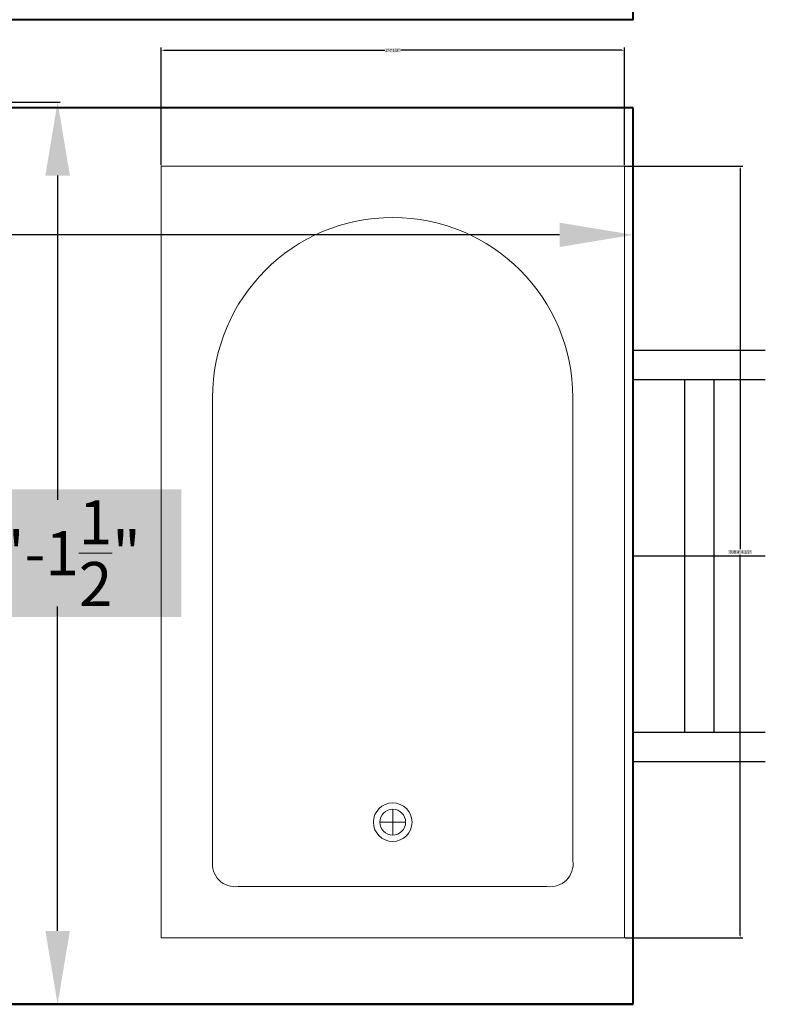
# Model space of a CAD drawing. Units: inches. Extents: x -301 to 715, y -607 to 364.
# Tile 98 of 141: x 82 to 133, y -77 to -10. Entities that reach past the tile are written whole.
import ezdxf

# ---------------------------------------------------------------- set-up
doc = ezdxf.new("R2010")
doc.units = ezdxf.units.IN
doc.header["$MEASUREMENT"] = 0
for name, color, linetype, lineweight in [('A-ANNO-DIMS', 2, 'Continuous', 18), ('A-FLOR-FIXT', 9, 'Continuous', 18), ('A-GLAZ', 2, 'Continuous', 25), ('A-WALL', 3, 'Continuous', 40)]:
    doc.layers.add(name, color=color, linetype=linetype, lineweight=lineweight)
doc.styles.get("Standard").update_dxf_attribs({"font": 'arial.ttf'})
doc.dimstyles.get("Standard").update_dxf_attribs({"dimtxt": 0.18, "dimasz": 0.18, "dimexe": 0.18, "dimexo": 0.0625, "dimgap": 0.09, "dimtad": 0, "dimtih": 1, "dimtoh": 1, "dimdec": 1, "dimzin": 0, "dimdsep": 46, "dimlunit": 4, "dimtxsty": 'Standard', "dimcen": 0.09, "dimclrd": 3, "dimclre": 4, "dimclrt": 6, "dimadec": 0, "dimazin": 0, "dimtfac": 1, "dimtdec": 1, "dimtofl": 0, "dimtmove": 0, "dimatfit": 3, "dimfxl": 1, "dimtfill": 2, "dimtfillclr": 51, "dimtolj": 1, "dimtzin": 0, "dimarcsym": 0})

# ---------------------------------------------------------------- blocks, each defined once
blk = doc.blocks.new('Bath Tub - 26 x 60 in.')
for p, q in [((9, -17), (9, -19)), ((8, -18), (10, -18))]:
    blk.add_line(p, q)
blk.add_lwpolyline([(0, -36), (0, 0), (60, 0), (60, -36)], close=True)
for points in [[(6, -4), (42, -4)], [(4, -30), (4, -6)], [(42, -32), (6, -32)]]:
    blk.add_lwpolyline(points)
for radius in [1.5, 1]:
    blk.add_circle((9, -18), radius)
for centre, radius, start, end in [((5.75, -5.75), 1.768, 81.8699, 188.1301), ((42, -18), 14, 270, 90), ((5.75, -30.25), 1.768, 171.8699, 278.1301)]:
    blk.add_arc(centre, radius, start, end)
blk = doc.blocks.new('*D46')
at = {"layer": 'A-ANNO-DIMS', "color": 0, "lineweight": -2, "transparency": 16777216}
for p, q in [((27.897, -15.88), (27.897, -24.639)), ((123.897, -15.88), (123.897, -24.639)), ((32.897, -24.459), (74.424, -24.459)), ((118.897, -24.459), (77.369, -24.459))]:
    blk.add_line(p, q, dxfattribs=at)
at = {"layer": 'A-ANNO-DIMS', "color": 0, "transparency": 16777216}
for points in [[(32.897, -23.626), (32.897, -25.292), (27.897, -24.459)], [(118.897, -23.626), (118.897, -25.292), (123.897, -24.459)]]:
    blk.add_solid(points, dxfattribs=at)
at = {"layer": 'Defpoints', "color": 0, "transparency": 16777216}
for p in [(27.897, -15.818), (123.897, -15.818), (123.897, -24.459)]:
    blk.add_point(p, dxfattribs=at)
at = {"layer": 'A-ANNO-DIMS', "color": 0, "transparency": 16777216, "insert": (75.897, -24.459), "char_height": 3, "attachment_point": 5, "bg_fill": 1, "box_fill_scale": 1.25, "bg_fill_color": 51, "bg_fill_transparency": 0}
blk.add_mtext("\\A1;8'", dxfattribs=at)
blk = doc.blocks.new('*D47')
at = {"layer": 'A-ANNO-DIMS', "color": 0, "lineweight": -2, "transparency": 16777216}
for p, q in [((53.666, -15.423), (84.935, -15.423)), ((84.755, -20.423), (84.755, -42.492)), ((84.755, -71.818), (84.755, -49.748)), ((57.415, -76.818), (84.935, -76.818))]:
    blk.add_line(p, q, dxfattribs=at)
at = {"layer": 'A-ANNO-DIMS', "color": 0, "transparency": 16777216}
for points in [[(83.922, -20.423), (85.588, -20.423), (84.755, -15.423)], [(83.922, -71.818), (85.588, -71.818), (84.755, -76.818)]]:
    blk.add_solid(points, dxfattribs=at)
at = {"layer": 'Defpoints', "color": 0, "transparency": 16777216}
for p in [(53.604, -15.423), (84.755, -15.423), (57.352, -76.818)]:
    blk.add_point(p, dxfattribs=at)
at = {"layer": 'A-ANNO-DIMS', "color": 0, "transparency": 16777216, "insert": (84.755, -46.12), "char_height": 3, "attachment_point": 5, "bg_fill": 1, "box_fill_scale": 1.25, "bg_fill_color": 51, "bg_fill_transparency": 0}
blk.add_mtext('\\A1;5\'-1{\\H1x;\\S1/2;}"', dxfattribs=at)
blk = doc.blocks.new('VENT-24-PLAN')
for p, q in [((0, 0), (0, 9)), ((2, 0), (2, 9)), ((14, 0), (14, 9)), ((26, 0), (26, 9)), ((28, 0), (28, 9)), ((26, 5.5), (2, 5.5)), ((26, 3.5), (2, 3.5))]:
    blk.add_line(p, q)
blk = doc.blocks.new('*D124')
at = {"layer": 'A-ANNO-DIMS', "color": 4, "lineweight": -2, "transparency": 16777216}
for p, q in [((123.372, -19.776), (131.368, -19.776)), ((123.372, -72.302), (131.368, -72.302))]:
    blk.add_line(p, q, dxfattribs=at)
at = {"layer": 'A-ANNO-DIMS', "color": 3, "lineweight": -2, "transparency": 16777216}
for p, q in [((131.188, -19.956), (131.188, -45.856)), ((131.188, -72.122), (131.188, -46.222))]:
    blk.add_line(p, q, dxfattribs=at)
at = {"layer": 'A-ANNO-DIMS', "color": 3, "transparency": 16777216}
for points in [[(131.158, -19.956), (131.218, -19.956), (131.188, -19.776)], [(131.158, -72.122), (131.218, -72.122), (131.188, -72.302)]]:
    blk.add_solid(points, dxfattribs=at)
at = {"layer": 'Defpoints', "color": 0, "transparency": 16777216}
for p in [(123.309, -19.776), (131.188, -19.776), (123.309, -72.302)]:
    blk.add_point(p, dxfattribs=at)
at = {"layer": 'A-ANNO-DIMS', "color": 6, "transparency": 16777216, "insert": (131.188, -46.039), "char_height": 0.18, "attachment_point": 5, "bg_fill": 1, "box_fill_scale": 1.25, "bg_fill_color": 51, "bg_fill_transparency": 0}
blk.add_mtext('\\A1;TUB 4\'-4 1/2"', dxfattribs=at)
blk = doc.blocks.new('*D125')
at = {"layer": 'A-ANNO-DIMS', "color": 4, "lineweight": -2, "transparency": 16777216}
for p, q in [((91.794, -19.714), (91.794, -11.718)), ((123.309, -19.714), (123.309, -11.718))]:
    blk.add_line(p, q, dxfattribs=at)
at = {"layer": 'A-ANNO-DIMS', "color": 3, "lineweight": -2, "transparency": 16777216}
for p, q in [((91.974, -11.898), (107.011, -11.898)), ((123.129, -11.898), (108.092, -11.898))]:
    blk.add_line(p, q, dxfattribs=at)
at = {"layer": 'A-ANNO-DIMS', "color": 3, "transparency": 16777216}
for points in [[(91.974, -11.868), (91.974, -11.928), (91.794, -11.898)], [(123.129, -11.868), (123.129, -11.928), (123.309, -11.898)]]:
    blk.add_solid(points, dxfattribs=at)
at = {"layer": 'Defpoints', "color": 0, "transparency": 16777216}
for p in [(91.794, -11.898), (91.794, -19.776), (123.309, -19.776)]:
    blk.add_point(p, dxfattribs=at)
at = {"layer": 'A-ANNO-DIMS', "color": 6, "transparency": 16777216, "insert": (107.551, -11.898), "char_height": 0.18, "attachment_point": 5, "bg_fill": 1, "box_fill_scale": 1.25, "bg_fill_color": 51, "bg_fill_transparency": 0}
blk.add_mtext('\\A1;2\'-7 1/2"', dxfattribs=at)

msp = doc.modelspace()

# ---------------------------------------------------------------- linework, layer by layer
at = {"layer": 'A-WALL'}
for p, q in [((123.897, -9.818), (123.897, 193.182)), ((123.897, -9.818), (21.897, -9.818)), ((123.897, -15.818), (27.897, -15.818)), ((123.897, -76.818), (123.897, -15.818)), ((57.352, -76.818), (123.897, -76.818)), ((123.897, -76.818), (75.897, -76.818))]:
    msp.add_line(p, q, dxfattribs=at)

# ---------------------------------------------------------------- block references
at = {"layer": 'A-FLOR-FIXT', "xscale": 0.875426725639565, "yscale": 0.875426725639565, "zscale": 0.875426725639565, "rotation": 90}
msp.add_blockref('Bath Tub - 26 x 60 in.', (91.794, -72.302), dxfattribs=at)
at = {"layer": 'A-GLAZ', "rotation": 89.99999999999955}
msp.add_blockref('VENT-24-PLAN', (132.897, -60.318), dxfattribs=at)

# ---------------------------------------------------------------- dimensions: what is measured, and where the dimension line sits
at = {"layer": 'A-ANNO-DIMS'}
for base, p1, p2, angle, override, picture, middle in [((91.794, -11.898), (123.309, -19.776), (91.794, -19.776), 180, {"dimdec": 1, "dimlfac": 1, "dimrnd": 0, "dimzin": 1, "dimdsep": 46, "dimlunit": 4, "dimfrac": 2}, '*D125', (107.551, -11.898)), ((84.755, -15.423), (57.352, -76.818), (53.604, -15.423), 90, {"dimtxt": 3, "dimasz": 5, "dimclrd": 0, "dimclre": 0, "dimclrt": 0}, '*D47', (84.755, -46.12))]:
    dim = msp.add_linear_dim(base=base, p1=p1, p2=p2, angle=angle, dimstyle='Standard', override=override, dxfattribs=at)
    dim.commit()
    dim.dimension.update_dxf_attribs({"geometry": picture, "text_midpoint": middle})
dim = msp.add_linear_dim(base=(123.897, -24.459), p1=(27.897, -15.818), p2=(123.897, -15.818), dimstyle='Standard', override={"dimtxt": 3, "dimasz": 5, "dimclrd": 0, "dimclre": 0, "dimclrt": 0}, dxfattribs=at)
dim.commit()
dim.dimension.update_dxf_attribs({"geometry": '*D46', "text_midpoint": (75.897, -24.459)})
dim = msp.add_linear_dim(base=(131.188, -19.776), p1=(123.309, -72.302), p2=(123.309, -19.776), angle=90, text='TUB <>', dimstyle='Standard', override={"dimdec": 1, "dimlfac": 1, "dimrnd": 0, "dimzin": 1, "dimdsep": 46, "dimlunit": 4, "dimfrac": 2}, dxfattribs=at)
dim.commit()
dim.dimension.update_dxf_attribs({"geometry": '*D124', "text_midpoint": (131.188, -46.039)})

doc.saveas('drawing.dxf')
